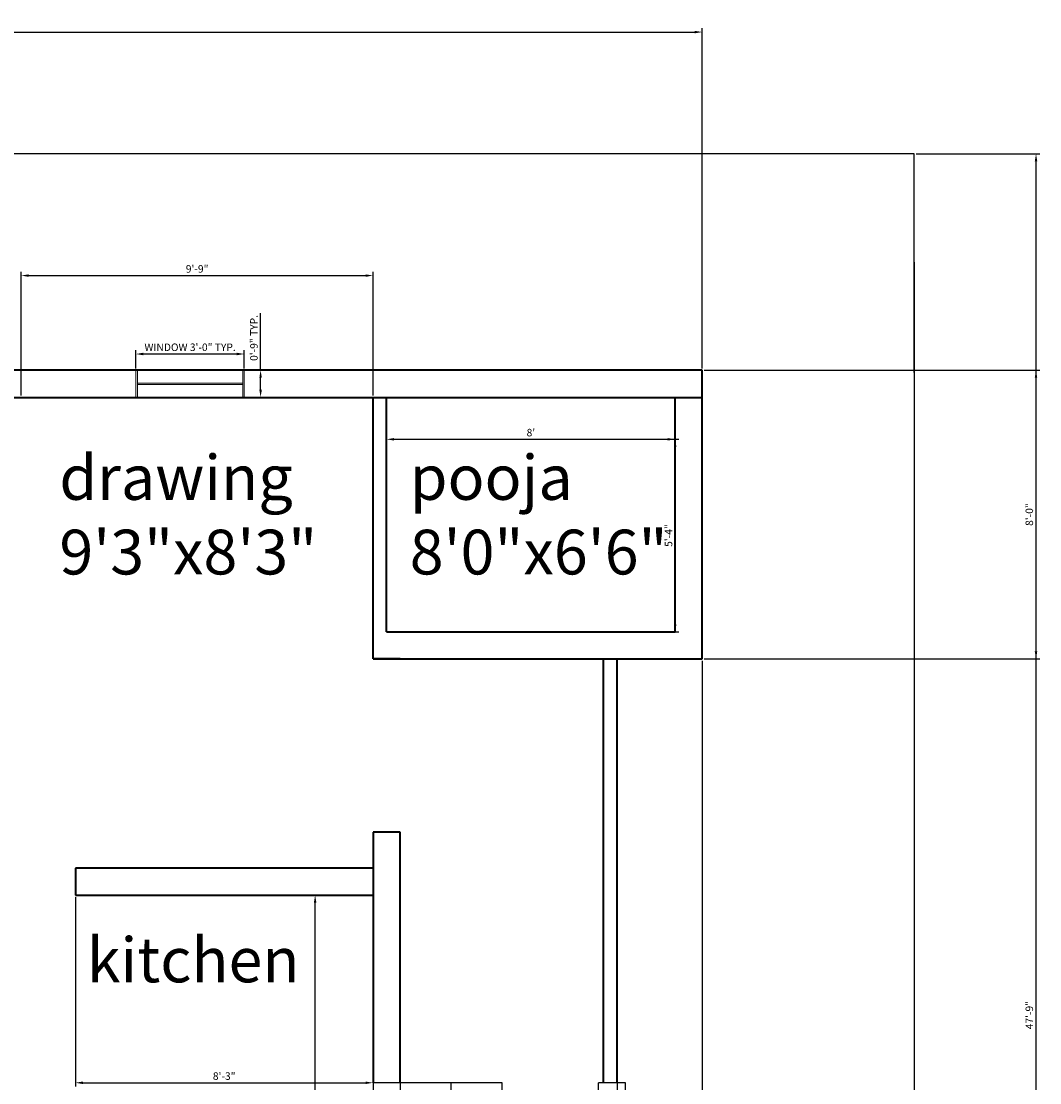
# Model space of a CAD drawing. Units: inches. Extents: x 250205121 to 250208111, y 89832590 to 89833271.
# Tile 9 of 14: x 250206724 to 250207062, y 89832906 to 89833259. Entities that reach past the tile are written whole.
import ezdxf

# ---------------------------------------------------------------- set-up
doc = ezdxf.new("R2010")
doc.units = ezdxf.units.IN
for name, color, linetype, lineweight in [('A-AREA-IDEN', 4, 'Continuous', 18), ('A-FLOR-STRS', 7, 'Continuous', 25), ('A-WALL', 7, 'Continuous', 35), ('C-PROP', 8, 'Continuous', 25), ('dimensions', 2, 'Continuous', 18), ('window', 4, 'Continuous', 18)]:
    doc.layers.add(name, color=color, linetype=linetype, lineweight=lineweight)
doc.styles.get("Standard").update_dxf_attribs({"font": 'arial.ttf'})
doc.dimstyles.new('ISO-25', dxfattribs={"dimtxt": 2.5, "dimasz": 2.5, "dimexe": 1.25, "dimexo": 0.625, "dimtad": 1, "dimlunit": 4, "dimtxsty": 'Standard', "dimcen": 2.5, "dimadec": 0, "dimazin": 0, "dimtfac": 1, "dimtmove": 0, "dimatfit": 3, "dimfxl": 1, "dimarcsym": 0})

# ---------------------------------------------------------------- blocks, each defined once
blk = doc.blocks.new('*D17')
at = {"layer": 'Defpoints', "color": 0, "transparency": 16777216}
for p in [(250206741.69, 89832968.74), (250206840.69, 89832968.74), (250206840.69, 89832906.33)]:
    blk.add_point(p, dxfattribs=at)
at = {"layer": 'dimensions', "color": 0, "lineweight": -2, "transparency": 16777216}
for p, q in [((250206741.69, 89832968.12), (250206741.69, 89832905.08)), ((250206840.69, 89832968.12), (250206840.69, 89832905.08)), ((250206744.19, 89832906.33), (250206838.19, 89832906.33))]:
    blk.add_line(p, q, dxfattribs=at)
at = {"layer": 'dimensions', "color": 0, "transparency": 16777216}
for points in [[(250206744.19, 89832906.74), (250206744.19, 89832905.91), (250206741.69, 89832906.33)], [(250206838.19, 89832906.74), (250206838.19, 89832905.91), (250206840.69, 89832906.33)]]:
    blk.add_solid(points, dxfattribs=at)
at = {"layer": 'dimensions', "color": 0, "transparency": 16777216, "insert": (250206791.19, 89832908.23), "char_height": 2.5, "attachment_point": 5}
blk.add_mtext('8\'-3"', dxfattribs=at)
blk = doc.blocks.new('*D18')
at = {"layer": 'Defpoints', "color": 0, "transparency": 16777216}
for p in [(250206821.44, 89832968.74), (250206823.27, 89832968.74), (250206823.27, 89832828.33)]:
    blk.add_point(p, dxfattribs=at)
at = {"layer": 'dimensions', "color": 0, "lineweight": -2, "transparency": 16777216}
for p, q in [((250206822.65, 89832968.74), (250206820.19, 89832968.74)), ((250206821.44, 89832830.83), (250206821.44, 89832966.24)), ((250206822.65, 89832828.33), (250206820.19, 89832828.33))]:
    blk.add_line(p, q, dxfattribs=at)
at = {"layer": 'dimensions', "color": 0, "transparency": 16777216}
for points in [[(250206821.02, 89832966.24), (250206821.85, 89832966.24), (250206821.44, 89832968.74)], [(250206821.02, 89832830.83), (250206821.85, 89832830.83), (250206821.44, 89832828.33)]]:
    blk.add_solid(points, dxfattribs=at)
at = {"layer": 'dimensions', "color": 0, "transparency": 16777216, "insert": (250206817.86, 89832898.53), "char_height": 2.5, "attachment_point": 5, "rotation": 90}
blk.add_mtext('11\'-8{\\H1x;\\S1/2;}"', dxfattribs=at)
blk = doc.blocks.new('*D19')
at = {"layer": 'Defpoints', "color": 0, "transparency": 16777216}
for p in [(250206941.19, 89833120.36), (250206845.19, 89833115.12), (250206941.19, 89833115.12)]:
    blk.add_point(p, dxfattribs=at)
at = {"layer": 'dimensions', "color": 0, "lineweight": -2, "transparency": 16777216}
for p, q in [((250206845.19, 89833115.74), (250206845.19, 89833121.61)), ((250206847.69, 89833120.36), (250206938.69, 89833120.36)), ((250206941.19, 89833115.74), (250206941.19, 89833121.61))]:
    blk.add_line(p, q, dxfattribs=at)
at = {"layer": 'dimensions', "color": 0, "transparency": 16777216}
for points in [[(250206847.69, 89833120.78), (250206847.69, 89833119.95), (250206845.19, 89833120.36)], [(250206938.69, 89833120.78), (250206938.69, 89833119.95), (250206941.19, 89833120.36)]]:
    blk.add_solid(points, dxfattribs=at)
at = {"layer": 'dimensions', "color": 0, "transparency": 16777216, "insert": (250206893.19, 89833122.26), "char_height": 2.5, "attachment_point": 5}
blk.add_mtext("8'", dxfattribs=at)
blk = doc.blocks.new('*D20')
at = {"layer": 'Defpoints', "color": 0, "transparency": 16777216}
for p in [(250206921.67, 89833120.36), (250206941.19, 89833120.36), (250206921.67, 89833056.33)]:
    blk.add_point(p, dxfattribs=at)
at = {"layer": 'dimensions', "color": 0, "lineweight": -2, "transparency": 16777216}
for p, q in [((250206922.29, 89833120.36), (250206942.44, 89833120.36)), ((250206941.19, 89833058.83), (250206941.19, 89833117.86)), ((250206922.29, 89833056.33), (250206942.44, 89833056.33))]:
    blk.add_line(p, q, dxfattribs=at)
at = {"layer": 'dimensions', "color": 0, "transparency": 16777216}
for points in [[(250206940.77, 89833117.86), (250206941.6, 89833117.86), (250206941.19, 89833120.36)], [(250206940.77, 89833058.83), (250206941.6, 89833058.83), (250206941.19, 89833056.33)]]:
    blk.add_solid(points, dxfattribs=at)
at = {"layer": 'dimensions', "color": 0, "transparency": 16777216, "insert": (250206939.29, 89833088.35), "char_height": 2.5, "attachment_point": 5, "rotation": 90}
blk.add_mtext('5\'-4"', dxfattribs=at)
blk = doc.blocks.new('WIN-36IN')
for p, q in [((0, 0), (0, 36.08)), ((0, 36.08), (9, 36.08)), ((0, 35.58), (9, 35.58)), ((4.3, 35.58), (4.3, 0.5)), ((4.7, 35.58), (4.7, 0.5)), ((9, 36.08), (9, 0)), ((9, 0.5), (0, 0.5)), ((9, 0), (0, 0))]:
    blk.add_line(p, q)
blk = doc.blocks.new('STAIR-RETURN')
for p, q in [((9, 192), (0, 192)), ((0, 192), (0, 0)), ((43, 192), (9, 192)), ((9, 192), (9, 0)), ((26, 23.7), (26, 192)), ((43, 36), (43, 192)), ((84, 192), (75, 192)), ((75, 0), (75, 192)), ((84, 156), (84, 192)), ((53.53, 184.53), (52.21, 185.69)), ((58.64, 180), (53.53, 184.53)), ((58.64, 180), (63.65, 185.66)), ((75, 180), (9, 180)), ((58.64, 180), (58.64, 23.7)), ((75, 168), (9, 168)), ((75, 156), (9, 156)), ((84, 156), (75, 156)), ((84, 152), (75, 152)), ((84, 116), (84, 152)), ((75, 144), (9, 144)), ((75, 132), (9, 132)), ((75, 120), (9, 120)), ((84, 116), (75, 116)), ((84, 112), (75, 112)), ((84, 76), (84, 112)), ((75, 108), (9, 108)), ((53.53, 106.37), (52.21, 107.54)), ((58.64, 101.85), (53.53, 106.37)), ((58.64, 101.85), (63.65, 107.51)), ((26, 101.85), (20.99, 96.18)), ((26, 101.85), (31.11, 97.32)), ((75, 96), (9, 96)), ((31.11, 97.32), (32.43, 96.16)), ((75, 84), (9, 84)), ((84, 76), (75, 76)), ((75, 72), (9, 72)), ((84, 72), (75, 72)), ((84, 0), (84, 72)), ((75, 60), (9, 60)), ((75, 48), (9, 48)), ((75, 36), (9, 36)), ((42.32, 23.7), (46.85, 28.81)), ((46.85, 28.81), (48.01, 30.12)), ((58.64, 23.7), (26, 23.7)), ((42.32, 23.7), (47.98, 18.68)), ((0, 9), (84, 9)), ((18, 0), (18, 9)), ((66, 0), (66, 9)), ((84, 9), (75, 9)), ((0, 0), (84, 0))]:
    blk.add_line(p, q)
blk = doc.blocks.new('*D33')
at = {"layer": 'Defpoints', "color": 0, "transparency": 16777216}
for p in [(250206761.8, 89833148.74), (250206761.8, 89833143.33), (250206797.88, 89833143.33)]:
    blk.add_point(p, dxfattribs=at)
at = {"layer": 'dimensions', "color": 0, "lineweight": -2, "transparency": 16777216}
for p, q in [((250206761.8, 89833143.95), (250206761.8, 89833149.99)), ((250206795.38, 89833148.74), (250206764.3, 89833148.74)), ((250206797.88, 89833143.95), (250206797.88, 89833149.99))]:
    blk.add_line(p, q, dxfattribs=at)
at = {"layer": 'dimensions', "color": 0, "transparency": 16777216}
for points in [[(250206764.3, 89833149.16), (250206764.3, 89833148.32), (250206761.8, 89833148.74)], [(250206795.38, 89833149.16), (250206795.38, 89833148.32), (250206797.88, 89833148.74)]]:
    blk.add_solid(points, dxfattribs=at)
at = {"layer": 'dimensions', "color": 0, "transparency": 16777216, "insert": (250206779.84, 89833150.66), "char_height": 2.5, "attachment_point": 5, "rotation": 360}
blk.add_mtext('WINDOW 3\'-0" TYP.', dxfattribs=at)
blk = doc.blocks.new('*D34')
at = {"layer": 'Defpoints', "color": 0, "transparency": 16777216}
for p in [(250206797.88, 89833143.33), (250206803.29, 89833143.33), (250206797.88, 89833134.33)]:
    blk.add_point(p, dxfattribs=at)
at = {"layer": 'dimensions', "color": 0, "lineweight": -2, "transparency": 16777216}
for p, q in [((250206803.29, 89833143.33), (250206803.29, 89833162.32)), ((250206798.51, 89833143.33), (250206804.54, 89833143.33)), ((250206803.29, 89833136.83), (250206803.29, 89833140.83)), ((250206798.51, 89833134.33), (250206804.54, 89833134.33))]:
    blk.add_line(p, q, dxfattribs=at)
at = {"layer": 'dimensions', "color": 0, "transparency": 16777216}
for points in [[(250206802.88, 89833140.83), (250206803.71, 89833140.83), (250206803.29, 89833143.33)], [(250206802.88, 89833136.83), (250206803.71, 89833136.83), (250206803.29, 89833134.33)]]:
    blk.add_solid(points, dxfattribs=at)
at = {"layer": 'dimensions', "color": 0, "transparency": 16777216, "insert": (250206801.39, 89833154.07), "char_height": 2.5, "attachment_point": 5, "rotation": 90}
blk.add_mtext('0\'-9" TYP.', dxfattribs=at)
blk = doc.blocks.new('*D55')
at = {"layer": 'Defpoints', "color": 0, "transparency": 16777216}
for p in [(250207020.69, 89833215.33), (250207061.19, 89833215.33), (250207020.69, 89832642.33)]:
    blk.add_point(p, dxfattribs=at)
at = {"layer": 'dimensions', "color": 0, "lineweight": -2, "transparency": 16777216}
for p, q in [((250207021.31, 89833215.33), (250207062.44, 89833215.33)), ((250207061.19, 89832644.83), (250207061.19, 89833212.83)), ((250207021.31, 89832642.33), (250207062.44, 89832642.33))]:
    blk.add_line(p, q, dxfattribs=at)
at = {"layer": 'dimensions', "color": 0, "transparency": 16777216}
for points in [[(250207060.77, 89833212.83), (250207061.6, 89833212.83), (250207061.19, 89833215.33)], [(250207060.77, 89832644.83), (250207061.6, 89832644.83), (250207061.19, 89832642.33)]]:
    blk.add_solid(points, dxfattribs=at)
at = {"layer": 'dimensions', "color": 0, "transparency": 16777216, "insert": (250207059.29, 89832928.83), "char_height": 2.5, "attachment_point": 5, "rotation": 90}
blk.add_mtext('47\'-9"', dxfattribs=at)
blk = doc.blocks.new('*D58')
at = {"layer": 'Defpoints', "color": 0, "transparency": 16777216}
for p in [(250206950.19, 89833255.83), (250206290.19, 89833143.33), (250206950.19, 89833143.33)]:
    blk.add_point(p, dxfattribs=at)
at = {"layer": 'dimensions', "color": 0, "lineweight": -2, "transparency": 16777216}
for p, q in [((250206290.19, 89833143.95), (250206290.19, 89833257.08)), ((250206292.69, 89833255.83), (250206947.69, 89833255.83)), ((250206950.19, 89833143.95), (250206950.19, 89833257.08))]:
    blk.add_line(p, q, dxfattribs=at)
at = {"layer": 'dimensions', "color": 0, "transparency": 16777216}
for points in [[(250206292.69, 89833256.24), (250206292.69, 89833255.41), (250206290.19, 89833255.83)], [(250206947.69, 89833256.24), (250206947.69, 89833255.41), (250206950.19, 89833255.83)]]:
    blk.add_solid(points, dxfattribs=at)
at = {"layer": 'dimensions', "color": 0, "transparency": 16777216, "insert": (250206620.19, 89833257.73), "char_height": 2.5, "attachment_point": 5}
blk.add_mtext('55\'-0"', dxfattribs=at)
blk = doc.blocks.new('*D62')
at = {"layer": 'Defpoints', "color": 0, "transparency": 16777216}
for p in [(250206921.85, 89833047.33), (250206950.19, 89833047.33), (250206950.19, 89832601.83)]:
    blk.add_point(p, dxfattribs=at)
at = {"layer": 'dimensions', "color": 0, "lineweight": -2, "transparency": 16777216}
for p, q in [((250206921.85, 89833046.7), (250206921.85, 89832600.58)), ((250206950.19, 89833046.7), (250206950.19, 89832600.58)), ((250206924.35, 89832601.83), (250206947.69, 89832601.83))]:
    blk.add_line(p, q, dxfattribs=at)
at = {"layer": 'dimensions', "color": 0, "transparency": 16777216}
for points in [[(250206924.35, 89832602.24), (250206924.35, 89832601.41), (250206921.85, 89832601.83)], [(250206947.69, 89832602.24), (250206947.69, 89832601.41), (250206950.19, 89832601.83)]]:
    blk.add_solid(points, dxfattribs=at)
at = {"layer": 'dimensions', "color": 0, "transparency": 16777216, "insert": (250206936.02, 89832603.75), "char_height": 2.5, "attachment_point": 5}
blk.add_mtext('2\'-4 1/2"', dxfattribs=at)
blk = doc.blocks.new('*D63')
at = {"layer": 'Defpoints', "color": 0, "transparency": 16777216}
for p in [(250206950.19, 89833143.33), (250207061.19, 89833143.33), (250206950.19, 89833047.33)]:
    blk.add_point(p, dxfattribs=at)
at = {"layer": 'dimensions', "color": 0, "lineweight": -2, "transparency": 16777216}
for p, q in [((250206950.81, 89833143.33), (250207062.44, 89833143.33)), ((250207061.19, 89833049.83), (250207061.19, 89833140.83)), ((250206950.81, 89833047.33), (250207062.44, 89833047.33))]:
    blk.add_line(p, q, dxfattribs=at)
at = {"layer": 'dimensions', "color": 0, "transparency": 16777216}
for points in [[(250207060.77, 89833140.83), (250207061.6, 89833140.83), (250207061.19, 89833143.33)], [(250207060.77, 89833049.83), (250207061.6, 89833049.83), (250207061.19, 89833047.33)]]:
    blk.add_solid(points, dxfattribs=at)
at = {"layer": 'dimensions', "color": 0, "transparency": 16777216, "insert": (250207059.29, 89833095.33), "char_height": 2.5, "attachment_point": 5, "rotation": 90}
blk.add_mtext('8\'-0"', dxfattribs=at)
blk = doc.blocks.new('*D64')
at = {"layer": 'Defpoints', "color": 0, "transparency": 16777216}
for p in [(250206840.69, 89833174.83), (250206723.69, 89833134.33), (250206840.69, 89833134.33)]:
    blk.add_point(p, dxfattribs=at)
at = {"layer": 'dimensions', "color": 0, "lineweight": -2, "transparency": 16777216}
for p, q in [((250206723.69, 89833134.95), (250206723.69, 89833176.08)), ((250206726.19, 89833174.83), (250206838.19, 89833174.83)), ((250206840.69, 89833134.95), (250206840.69, 89833176.08))]:
    blk.add_line(p, q, dxfattribs=at)
at = {"layer": 'dimensions', "color": 0, "transparency": 16777216}
for points in [[(250206726.19, 89833175.24), (250206726.19, 89833174.41), (250206723.69, 89833174.83)], [(250206838.19, 89833175.24), (250206838.19, 89833174.41), (250206840.69, 89833174.83)]]:
    blk.add_solid(points, dxfattribs=at)
at = {"layer": 'dimensions', "color": 0, "transparency": 16777216, "insert": (250206782.19, 89833176.73), "char_height": 2.5, "attachment_point": 5}
blk.add_mtext('9\'-9"', dxfattribs=at)

msp = doc.modelspace()

# ---------------------------------------------------------------- linework, layer by layer
at = {"layer": 'A-WALL'}
for p, q in [((250206950.187, 89833143.328), (250206299.187, 89833143.328)), ((250206950.187, 89833047.328), (250206950.187, 89833143.328)), ((250206299.187, 89833134.328), (250206950.187, 89833134.328)), ((250206840.687, 89833047.328), (250206840.687, 89833134.328)), ((250206845.187, 89833056.328), (250206845.187, 89833134.328)), ((250206941.187, 89833056.328), (250206941.187, 89833134.328)), ((250206845.187, 89833056.328), (250206941.187, 89833056.328)), ((250206840.687, 89833047.328), (250206950.187, 89833047.328)), ((250206849.687, 89833047.328), (250206840.687, 89833047.328)), ((250206917.347, 89832906.328), (250206917.347, 89833047.328)), ((250206921.847, 89832906.328), (250206921.847, 89833047.328)), ((250206849.687, 89832989.74), (250206840.687, 89832989.74)), ((250206840.687, 89832989.74), (250206840.687, 89832906.328)), ((250206840.687, 89832989.74), (250206840.687, 89832977.74)), ((250206849.687, 89832906.328), (250206849.687, 89832989.74)), ((250206840.687, 89832977.74), (250206741.687, 89832977.74)), ((250206741.687, 89832977.74), (250206741.687, 89832968.74)), ((250206741.687, 89832968.74), (250206840.687, 89832968.74))]:
    msp.add_line(p, q, dxfattribs=at)
at = {"layer": 'C-PROP'}
for p, q in [((250207020.687, 89833215.328), (250206543.687, 89833215.328)), ((250207020.687, 89833179.328), (250207020.687, 89833215.328)), ((250207020.687, 89833142.574), (250207020.687, 89833179.328)), ((250207020.687, 89833179.328), (250207020.687, 89832642.328)), ((250207020.687, 89832978.328), (250207020.687, 89832978.328))]:
    msp.add_line(p, q, dxfattribs=at)

# ---------------------------------------------------------------- block references
at = {"layer": 'A-FLOR-STRS'}
msp.add_blockref('STAIR-RETURN', (250206840.687, 89832714.328), dxfattribs=at)
at = {"layer": 'window', "rotation": 89.99999987754511}
msp.add_blockref('WIN-36IN', (250206797.883, 89833134.328), dxfattribs=at)

# ---------------------------------------------------------------- texts
at = {"layer": 'A-AREA-IDEN', "char_height": 14.8861, "attachment_point": 1}
for s, insert in [('drawing\\P9\'3"x8\'3"', (250206736.364, 89833115.116)), ('pooja\\P8\'0"x6\'6"', (250206852.89, 89833115.116)), ('kitchen', (250206745.484, 89832954.628))]:
    msp.add_mtext_dynamic_manual_height_columns(s, width=23.63705, gutter_width=74.43, heights=[0], dxfattribs=dict(at, insert=insert))

# ---------------------------------------------------------------- dimensions: what is measured, and where the dimension line sits
at = {"layer": 'dimensions'}
for base, p1, p2, override, picture, middle in [((250206950.187, 89833255.828), (250206290.187, 89833143.328), (250206950.187, 89833143.328), {"dimdec": 1, "dimlfac": 1, "dimrnd": 0, "dimzin": 1, "dimdsep": 46, "dimlunit": 4, "dimfrac": 2}, '*D58', (250206620.187, 89833257.729)), ((250206941.187, 89833120.363), (250206845.187, 89833115.116), (250206941.187, 89833115.116), {"dimclrd": 0, "dimclre": 0, "dimclrt": 0}, '*D19', (250206893.187, 89833122.265)), ((250206950.187, 89832601.828), (250206921.847, 89833047.328), (250206950.187, 89833047.328), {"dimdec": 1, "dimlfac": 1, "dimrnd": 0, "dimzin": 1, "dimdsep": 46, "dimlunit": 4, "dimfrac": 2}, '*D62', (250206936.017, 89832603.746)), ((250206840.687, 89832906.328), (250206741.687, 89832968.74), (250206840.687, 89832968.74), {"dimclrd": 0, "dimclre": 0, "dimclrt": 0}, '*D17', (250206791.187, 89832908.23))]:
    dim = msp.add_linear_dim(base=base, p1=p1, p2=p2, dimstyle='ISO-25', override=override, dxfattribs=at)
    dim.commit()
    dim.dimension.update_dxf_attribs({"geometry": picture, "text_midpoint": middle})
for base, p1, p2, angle, override, picture, middle in [((250207061.187, 89833215.328), (250207020.687, 89832642.328), (250207020.687, 89833215.328), 90, {"dimdec": 1, "dimlfac": 1, "dimrnd": 0, "dimzin": 1, "dimdsep": 46, "dimlunit": 4, "dimfrac": 2}, '*D55', (250207059.286, 89832928.828)), ((250206840.687, 89833174.828), (250206723.687, 89833134.328), (250206840.687, 89833134.328), 360, {"dimdec": 1, "dimlfac": 1, "dimrnd": 0, "dimzin": 1, "dimdsep": 46, "dimlunit": 4, "dimfrac": 2}, '*D64', (250206782.187, 89833176.729)), ((250207061.187, 89833143.328), (250206950.187, 89833047.328), (250206950.187, 89833143.328), 90, {"dimdec": 1, "dimlfac": 1, "dimrnd": 0, "dimzin": 1, "dimdsep": 46, "dimlunit": 4, "dimfrac": 2}, '*D63', (250207059.286, 89833095.328)), ((250206941.1872, 89833120.3635), (250206921.6655, 89833056.328), (250206921.6655, 89833120.3635), 90, {"dimclrd": 0, "dimclre": 0, "dimclrt": 0}, '*D20', (250206939.2909, 89833088.3457)), ((250206821.437, 89832968.74), (250206823.271, 89832828.328), (250206823.271, 89832968.74), 90, {"dimclrd": 0, "dimclre": 0, "dimclrt": 0}, '*D18', (250206817.864, 89832898.534))]:
    dim = msp.add_linear_dim(base=base, p1=p1, p2=p2, angle=angle, dimstyle='ISO-25', override=override, dxfattribs=at)
    dim.commit()
    dim.dimension.update_dxf_attribs({"geometry": picture, "text_midpoint": middle})
for base, p1, p2, angle, text, picture, middle in [((250206803.295, 89833143.328), (250206797.883, 89833134.328), (250206797.883, 89833143.328), 90, '<> TYP.', '*D34', (250206801.393, 89833154.072)), ((250206761.804, 89833148.74), (250206797.883, 89833143.328), (250206761.804, 89833143.328), 180, 'WINDOW <> TYP.', '*D33', (250206779.843, 89833150.659))]:
    dim = msp.add_linear_dim(base=base, p1=p1, p2=p2, angle=angle, text=text, dimstyle='ISO-25', override={"dimdec": 1, "dimlfac": 1, "dimrnd": 0, "dimzin": 1, "dimdsep": 46, "dimlunit": 4, "dimfrac": 2}, dxfattribs=at)
    dim.commit()
    dim.dimension.update_dxf_attribs({"geometry": picture, "text_midpoint": middle})

doc.saveas('drawing.dxf')
